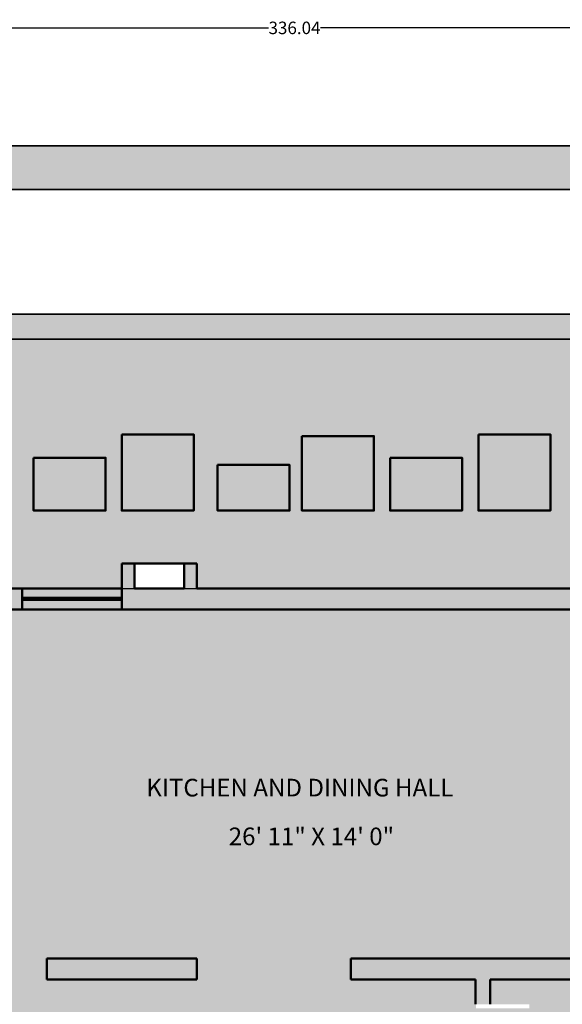
# Model space of a CAD drawing. Units: inches. Extents: x 925 to 2834, y 111 to 1355.
# Tile 17 of 25: x 1293 to 1553, y 882 to 1355. Entities that reach past the tile are written whole.
import ezdxf

# ---------------------------------------------------------------- set-up
doc = ezdxf.new("R2010")
doc.units = ezdxf.units.IN
doc.header["$MEASUREMENT"] = 0
for name, color, linetype, lineweight in [('A-ANNO-DIMS', 2, 'Continuous', 18), ('A-ANNO-TTLB', 7, 'Continuous', 35), ('A-AREA-IDEN', 7, 'Continuous', 18), ('A-FLOR-PATT', 252, 'Continuous', 13), ('A-GLAZ', 3, 'Continuous', 25), ('A-WALL', 7, 'Continuous', 50), ('A-WALL-PATT', 8, 'Continuous', 13)]:
    doc.layers.add(name, color=color, linetype=linetype, lineweight=lineweight)
doc.styles.get("Standard").update_dxf_attribs({"font": 'arial.ttf'})
doc.dimstyles.get("Standard").update_dxf_attribs({"dimtxt": 6, "dimasz": 3, "dimexe": 0.18, "dimexo": 0.0625, "dimgap": 0.09, "dimtad": 0, "dimtih": 1, "dimtoh": 1, "dimdec": 1, "dimzin": 0, "dimdsep": 46, "dimlunit": 3, "dimtxsty": 'Standard', "dimblk": 'ARCHTICK', "dimcen": 0.09, "dimadec": 0, "dimazin": 0, "dimtfac": 1, "dimtdec": 1, "dimtofl": 0, "dimtmove": 0, "dimatfit": 3, "dimfxl": 1, "dimtolj": 1, "dimtzin": 0, "dimarcsym": 0})

# ---------------------------------------------------------------- blocks, each defined once
blk = doc.blocks.new('_ArchTick')
at = {"color": 0, "linetype": 'ByBlock', "const_width": 0.15}
blk.add_lwpolyline([(-0.5, -0.5), (0.5, 0.5)], dxfattribs=at)
blk = doc.blocks.new('*D16')
at = {"layer": 'A-ANNO-DIMS', "color": 0, "lineweight": -2, "transparency": 16777216}
for p, q in [((1256.67, 1081.65), (1256.67, 1351.49)), ((1256.67, 1351.31), (1412.16, 1351.31)), ((1592.71, 1351.31), (1437.22, 1351.31)), ((1592.71, 1071.65), (1592.71, 1351.49))]:
    blk.add_line(p, q, dxfattribs=at)
at = {"layer": 'Defpoints', "color": 0, "transparency": 16777216}
for p in [(1592.71, 1351.31), (1256.67, 1081.59), (1592.71, 1071.59)]:
    blk.add_point(p, dxfattribs=at)
at = {"layer": 'A-ANNO-DIMS', "color": 0, "lineweight": -2, "transparency": 16777216, "xscale": 3, "yscale": 3, "zscale": 3, "rotation": 180}
blk.add_blockref('_ArchTick', (1256.67, 1351.31), dxfattribs=at)
at = {"layer": 'A-ANNO-DIMS', "color": 0, "lineweight": -2, "transparency": 16777216, "xscale": 3, "yscale": 3, "zscale": 3}
blk.add_blockref('_ArchTick', (1592.71, 1351.31), dxfattribs=at)
at = {"layer": 'A-ANNO-DIMS', "color": 0, "transparency": 16777216, "insert": (1424.69, 1351.31), "char_height": 6, "attachment_point": 5}
blk.add_mtext('\\A1;336.04', dxfattribs=at)

msp = doc.modelspace()

# ---------------------------------------------------------------- hatches: boundary and pattern name
at = {"layer": 'A-FLOR-PATT', "transparency": 33554605}
h = msp.add_hatch(color=256, dxfattribs=at)
h.dxf.hatch_style = 1
h.paths.add_polyline_path([(1931.688, 1294.5638), (991.7375, 1294.5638), (991.7375, 172.1134), (1931.688, 172.1134)])
h.paths.add_polyline_path([(1910.7128, 1273.5886), (1910.7128, 193.0886), (1012.7128, 193.0886), (1012.7128, 1273.5886)], flags=16)
h.paths.add_polyline_path([(1850.7128, 1213.5886), (1850.7128, 253.0886), (1072.7128, 253.0886), (1072.7128, 1213.5886)], flags=0)
h.paths.add_polyline_path([(1838.7128, 1201.5886), (1838.7128, 265.0886), (1084.7128, 265.0886), (1084.7128, 530.5886), (1084.7128, 1201.5886)], flags=0)
h.paths.add_polyline_path([(1547.6758, 1155.7396), (1547.6758, 1119.115), (1513.0687, 1119.115), (1513.0687, 1155.7396)], flags=0)
h.paths.add_polyline_path([(1600.1067, 1154.9439), (1634.7139, 1154.9439), (1634.7139, 1119.115), (1600.1067, 1119.115)], flags=0)
h.paths.add_polyline_path([(1505.2502, 1144.5358), (1505.2502, 1119.115), (1470.643, 1119.115), (1470.643, 1144.5358)], flags=0)
h.paths.add_polyline_path([(1559.1357, 1141.0962), (1593.7428, 1141.0962), (1593.7428, 1119.115), (1559.1357, 1119.115)], flags=0)
h.paths.add_polyline_path([(1462.8966, 1154.9439), (1462.8966, 1119.115), (1428.2895, 1119.115), (1428.2895, 1154.9439)], flags=0)
h.paths.add_polyline_path([(1642.4603, 1144.5358), (1677.0675, 1144.5358), (1677.0675, 1119.115), (1642.4603, 1119.115)], flags=0)
h.paths.add_polyline_path([(1422.3508, 1141.0962), (1422.3508, 1119.115), (1387.7436, 1119.115), (1387.7436, 1141.0962)], flags=0)
h.paths.add_polyline_path([(1684.8859, 1155.7396), (1719.4931, 1155.7396), (1719.4931, 1119.115), (1684.8859, 1119.115)], flags=0)
h.paths.add_polyline_path([(1718.7128, 1081.5886), (1718.7128, 1050.1249), (1715.7128, 1050.1249), (1715.7128, 1026.1249), (1715.7128, 1002.1249), (1718.7128, 1002.1249), (1730.7128, 1002.1249), (1730.7128, 998.1249), (1730.7128, 990.1249), (1730.7128, 986.1249), (1718.7128, 986.1249), (1718.7128, 893.5886), (1715.3735, 893.5886), (1715.3735, 891.5886), (1713.3735, 891.5886, 0.41421356), (1677.3735, 855.5886), (1713.3735, 855.5886), (1713.3735, 853.5886), (1715.3735, 853.5886), (1715.3735, 851.5886), (1718.7128, 851.5886), (1718.7128, 821.5865), (1734.4655, 821.5865), (1734.3735, 819.5886, -0.41421356), (1712.4415, 793.5886), (1712.4415, 791.5886), (1718.7128, 791.5886), (1718.7128, 717.5886), (1718.7128, 669.5886), (1732.7128, 669.5886), (1732.7128, 665.5886), (1732.7128, 641.5886), (1732.7128, 634.5886), (1732.7128, 610.5886), (1732.7128, 603.5886), (1718.7128, 603.5886), (1718.7128, 385.0886), (1434.2128, 385.0886), (1434.2128, 530.5886), (1410.2128, 530.5886), (1408.2128, 530.5886), (1408.2128, 532.5886, 0.41421356), (1372.2128, 568.5886), (1372.2128, 532.5886), (1370.2128, 532.5886), (1370.2128, 530.5886), (1368.2128, 530.5886), (1282.2128, 530.5886), (1210.2128, 530.5886), (1200.2128, 530.5886), (1200.2128, 542.1915), (1183.2307, 542.1915), (1183.2307, 546.1915), (1200.2128, 546.1915), (1200.2128, 572.1915), (1183.2307, 572.1915), (1183.2307, 576.1915), (1200.2128, 576.1915), (1200.2128, 727.5886), (1210.2128, 727.5886), (1234.2128, 727.5886), (1259.7128, 727.5886), (1259.7128, 775.5886), (1259.7128, 799.5886), (1259.7128, 847.5886), (1259.7128, 993.5872), (1259.7128, 1065.5872), (1259.7128, 1071.5886), (1219.6318, 1071.5886), (1219.6318, 1081.5886), (1084.7128, 1081.5886), (1084.7128, 1119.115), (1256.8974, 1119.115), (1256.8974, 1154.9439), (1291.5046, 1154.9439), (1291.5046, 1119.115), (1256.8974, 1119.115), (1256.6723, 1081.5886), (1293.7128, 1081.5886), (1341.7128, 1081.5886), (1341.7128, 1093.5886), (1347.7128, 1093.5886), (1371.7128, 1093.5886), (1377.7128, 1093.5886), (1377.7128, 1081.5886), (1668.7128, 1081.5886), (1668.7128, 1117.5886), (1675.7128, 1117.5886), (1711.7128, 1117.5886), (1718.7128, 1117.5886)], flags=0)
h.paths.add_polyline_path([(1376.2838, 1155.7396), (1376.2838, 1119.115), (1341.6766, 1119.115), (1341.6766, 1155.7396)], flags=0)
h.paths.add_polyline_path([(1341.7128, 1076.0886), (1293.7128, 1076.0886), (1293.7128, 1071.5886), (1269.7128, 1071.5886), (1269.7128, 1065.5872), (1266.7128, 1065.5872), (1266.7128, 1029.5872), (1265.7128, 1029.5872), (1265.7128, 993.5872), (1269.7128, 993.5872), (1269.7128, 903.5886), (1269.7128, 893.5886), (1269.7128, 847.5886), (1265.2128, 847.5886), (1265.2128, 799.5886), (1269.7128, 799.5886), (1269.7128, 775.5886), (1265.2128, 775.5886), (1265.2128, 727.5886), (1269.7128, 727.5886), (1444.2128, 727.5886), (1444.2128, 717.5886), (1234.2128, 717.5886), (1234.2128, 722.0886), (1210.2128, 722.0886), (1210.2128, 717.5886), (1210.2128, 540.5886), (1210.2128, 536.0886), (1282.2128, 536.0886), (1282.2128, 535.0886), (1210.2128, 535.0886), (1210.2128, 540.5886), (1210.2128, 717.5886), (1210.2128, 723.0886), (1234.2128, 723.0886), (1234.2128, 717.5886), (1444.2128, 717.5886), (1444.2128, 727.5886), (1269.7128, 727.5886), (1264.2128, 727.5886), (1264.2128, 775.5886), (1269.7128, 775.5886), (1269.7128, 799.5886), (1264.2128, 799.5886), (1264.2128, 847.5886), (1269.7128, 847.5886), (1269.7128, 893.5886), (1269.7128, 903.5886), (1269.7128, 993.5872), (1264.7128, 993.5872), (1264.7128, 1029.5872), (1265.7128, 1029.5872), (1265.7128, 1065.5872), (1269.7128, 1065.5872), (1269.7128, 1071.5886), (1293.7128, 1071.5886), (1293.7128, 1077.0886), (1341.7128, 1077.0886)], flags=0)
h.paths.add_polyline_path([(1730.9529, 1141.0962), (1765.5601, 1141.0962), (1765.5601, 1119.115), (1730.9529, 1119.115)], flags=0)
h.paths.add_polyline_path([(1333.8582, 1144.5358), (1333.8582, 1119.115), (1299.251, 1119.115), (1299.251, 1144.5358)], flags=0)
h.paths.add_polyline_path([(1592.7128, 968.5886), (1596.0342, 968.5886), (1602.7128, 968.5886), (1708.7128, 968.5886), (1708.7128, 903.5886), (1602.7128, 903.5886), (1602.7128, 938.5886), (1592.7128, 938.5886), (1592.7128, 903.5886), (1451.7128, 903.5886), (1451.7128, 893.5886), (1511.7128, 893.5886), (1511.7128, 881.5886), (1515.2128, 881.5886), (1518.7128, 881.5886), (1518.7128, 893.5886), (1592.7128, 893.5886), (1592.7128, 799.5886), (1518.7128, 799.5886), (1518.7128, 857.5886), (1511.7128, 857.5886), (1511.7128, 799.5886), (1511.7128, 772.0886), (1521.7128, 772.0886), (1521.7128, 792.5886), (1592.7128, 792.5886), (1592.7128, 727.5886), (1521.7128, 727.5886), (1521.7128, 748.0886), (1511.7128, 748.0886), (1511.7128, 717.5886), (1708.7128, 717.5886), (1714.2128, 717.5886), (1714.2128, 669.5886), (1708.7128, 669.5886), (1708.7128, 641.5886), (1492.2128, 641.5886), (1492.2128, 631.5886), (1621.2128, 631.5886), (1621.2128, 443.0886), (1625.7128, 443.0886), (1625.7128, 503.0886), (1625.7128, 507.5886), (1625.7128, 631.5886), (1708.7128, 631.5886), (1708.7128, 507.5886), (1655.7128, 507.5886), (1655.7128, 503.0886), (1708.7128, 503.0886), (1708.7128, 395.0886), (1625.7128, 395.0886), (1625.7128, 419.0886), (1621.2128, 419.0886), (1621.2128, 395.0886), (1482.2128, 395.0886), (1482.2128, 385.0886), (1434.2128, 385.0886), (1434.2128, 433.0886), (1444.2128, 433.0886), (1444.2128, 631.5886), (1450.2128, 631.5886), (1450.2128, 634.91), (1452.2128, 634.91), (1452.2128, 669.5886), (1454.2128, 669.5886, -0.40021217), (1490.1712, 635.3173), (1492.2128, 635.3173), (1492.2128, 641.5886), (1564.7128, 641.5886), (1564.7128, 677.5886), (1672.7128, 677.5886), (1672.7128, 681.5886), (1564.7128, 681.5886), (1564.7128, 717.5886), (1511.7128, 717.5886), (1511.7128, 748.0886), (1511.7128, 772.0886), (1511.7128, 799.5886), (1511.7128, 857.5886), (1511.8913, 857.5886), (1511.8913, 859.5886), (1515.6201, 859.5886, 0.41421356), (1537.552, 879.5886), (1513.552, 879.5886), (1511.8913, 879.5886), (1511.8913, 881.5886), (1511.7128, 881.5886), (1511.7128, 893.5886), (1451.7128, 893.5886), (1451.7128, 903.5886), (1592.7128, 903.5886), (1592.7128, 938.5886), (1592.7128, 940.5886), (1596.4415, 940.5886, 0.41421356), (1618.3735, 966.5886), (1594.3735, 966.5886), (1592.7128, 966.5886)], flags=0)
h.paths.add_polyline_path([(1377.7128, 903.5886), (1377.7128, 893.5886), (1305.7128, 893.5886), (1305.7128, 903.5886)], flags=0)
h.paths.add_polyline_path([(1708.7128, 821.5886), (1712.0342, 821.5886), (1712.0342, 819.5886), (1710.3735, 819.5886), (1708.7128, 819.5886)], flags=0)
h.paths.add_polyline_path([(1576.7128, 695.1992), (1575.5896, 693.6649), (1575.9687, 694.6994), (1575.4438, 695.1992), (1575.9687, 695.699), (1575.5896, 696.7335)], flags=0)
h.paths.add_polyline_path([(1565.9817, 662.3134), (1565.4568, 661.8136), (1565.8359, 660.7791), (1564.7128, 662.3134), (1565.8359, 663.8477), (1565.4568, 662.8132)], flags=0)
h.paths.add_polyline_path([(1444.2128, 433.0886), (1444.2128, 395.0886), (1482.2128, 395.0886), (1482.2128, 389.0886), (1438.2128, 389.0886), (1438.2128, 391.8608), (1438.2128, 433.0886)], flags=0)
h.paths.add_polyline_path([(1410.2128, 506.5886), (1410.2128, 289.0886), (1108.7128, 289.0886), (1108.7128, 506.5886)], flags=0)
h.paths.add_polyline_path([(1612.3153, 838.3016), (1680.4151, 838.3016), (1680.4151, 851.3131), (1612.3153, 851.3131)], flags=8)
h.paths.add_polyline_path([(1208.3174, 395.0436), (1282.1017, 395.0436), (1282.1017, 408.0552), (1208.3174, 408.0552)], flags=8)
h.paths.add_polyline_path([(1291.8049, 598.7427), (1369.8017, 598.7427), (1369.8017, 611.7542), (1291.8049, 611.7542)], flags=8)
h.paths.add_polyline_path([(1119.679, 917.3022), (1191.0817, 917.3022), (1191.0817, 930.3137), (1119.679, 930.3137)], flags=8)
h.paths.add_polyline_path([(1332.2261, 815.9808), (1410.2258, 815.9808), (1410.2258, 829.001), (1332.2261, 829.001)], flags=8)
h.paths.add_polyline_path([(1390.9013, 955.8158), (1475.4981, 955.8158), (1475.4981, 968.8273), (1390.9013, 968.8273)], flags=8)
h.paths.add_polyline_path([(1620.3436, 998.9325), (1688.4434, 998.9325), (1688.4434, 1011.944), (1620.3436, 1011.944)], flags=8)
h.paths.add_polyline_path([(1620.3436, 914.1039), (1691.7405, 914.1039), (1691.7405, 927.1155), (1620.3436, 927.1155)], flags=8)
h.paths.add_polyline_path([(1521.4542, 816.005), (1589.5569, 816.005), (1589.5569, 829.0253), (1521.4542, 829.0253)], flags=8)
h.paths.add_polyline_path([(1528.524, 740.3497), (1602.3082, 740.3497), (1602.3082, 753.3613), (1528.524, 753.3613)], flags=8)
h.paths.add_polyline_path([(1627.6094, 762.6128), (1702.3091, 762.6128), (1702.3091, 775.6244), (1627.6094, 775.6244)], flags=8)
h.paths.add_polyline_path([(1610.5442, 657.2751), (1684.3284, 657.2751), (1684.3284, 670.2867), (1610.5442, 670.2867)], flags=8)
h.paths.add_polyline_path([(1636.6983, 519.472), (1711.3981, 519.472), (1711.3981, 532.4835), (1636.6983, 532.4835)], flags=8)
h.paths.add_polyline_path([(1616.8577, 424.8539), (1694.8545, 424.8539), (1694.8545, 437.8654), (1616.8577, 437.8654)], flags=8)
h.paths.add_polyline_path([(1506.1456, 460.8838), (1579.9299, 460.8838), (1579.9299, 473.8953), (1506.1456, 473.8953)], flags=8)
h.paths.add_polyline_path([(1624.6119, 784.6011), (1696.9185, 784.6011), (1696.9185, 797.7864), (1624.6119, 797.7864)], flags=8)
h.paths.add_polyline_path([(1606.3732, 854.2194), (1683.3039, 854.2194), (1683.3039, 867.4048), (1606.3732, 867.4048)], flags=8)
h.paths.add_polyline_path([(1127.8008, 940.3581), (1165.1637, 940.3581), (1165.1637, 953.5348), (1127.8008, 953.5348)], flags=8)
h.paths.add_polyline_path([(1620.8657, 1019.4968), (1677.3447, 1019.4968), (1677.3447, 1032.6735), (1620.8657, 1032.6735)], flags=8)
h.paths.add_polyline_path([(1620.8643, 930.1821), (1703.0564, 930.1821), (1703.0564, 943.3675), (1620.8643, 943.3675)], flags=8)
h.paths.add_polyline_path([(1324.5702, 836.8338), (1408.0892, 836.8338), (1408.0892, 850.0191), (1324.5702, 850.0191)], flags=8)
h.paths.add_polyline_path([(1281.6584, 622.8885), (1383.6213, 622.8885), (1383.6213, 636.0739), (1281.6584, 636.0739)], flags=8)
h.paths.add_polyline_path([(1210.6721, 416.7893), (1269.1299, 416.7893), (1269.1299, 429.9747), (1210.6721, 429.9747)], flags=8)
h.paths.add_polyline_path([(1507.8264, 477.4836), (1586.7329, 477.4836), (1586.7329, 490.669), (1507.8264, 490.669)], flags=8)
h.paths.add_polyline_path([(1643.6238, 443.8135), (1696.6696, 443.8135), (1696.6696, 456.5643), (1643.6238, 456.5643)], flags=8)
h.paths.add_polyline_path([(1647.2466, 540.5638), (1693.1825, 540.5638), (1693.1825, 553.7491), (1647.2466, 553.7491)], flags=8)
h.paths.add_polyline_path([(1626.0633, 668.5064), (1673.3174, 668.5064), (1673.3174, 681.6831), (1626.0633, 681.6831)], flags=8)
h.paths.add_polyline_path([(1538.2915, 830.7872), (1567.5942, 830.7872), (1567.5942, 843.5293), (1538.2915, 843.5293)], flags=8)
h.paths.add_polyline_path([(1530.9338, 754.0477), (1559.576, 754.0477), (1559.576, 766.7898), (1530.9338, 766.7898)], flags=8)
h.paths.add_polyline_path([(1351.2461, 979.2309), (1513.8919, 979.2309), (1513.8919, 992.4076), (1351.2461, 992.4076)], flags=8)
at = {"layer": 'A-FLOR-PATT'}
h = msp.add_hatch(color=256, dxfattribs=at)
h.dxf.hatch_style = 1
h.paths.add_polyline_path([(1850.7128, 1213.5886), (1072.7128, 1213.5886), (1072.7128, 253.0886), (1850.7128, 253.0886)])
h.paths.add_polyline_path([(1084.7128, 1201.5886), (1838.7128, 1201.5886), (1838.7128, 265.0886), (1084.7128, 265.0886)], flags=16)
h.paths.add_polyline_path([(1183.2307, 576.1915), (1200.2128, 576.1915), (1200.2128, 727.5886), (1210.2128, 727.5886), (1234.2128, 727.5886), (1259.7128, 727.5886), (1259.7128, 775.5886), (1259.7128, 799.5886), (1259.7128, 847.5886), (1259.7128, 993.5872), (1259.7128, 1065.5872), (1259.7128, 1071.5886), (1219.6318, 1071.5886), (1219.6318, 1081.5886), (1293.7128, 1081.5886), (1341.7128, 1081.5886), (1341.7128, 1093.5886), (1347.7128, 1093.5886), (1347.7128, 1081.5886), (1371.7128, 1081.5886), (1371.7128, 1093.5886), (1377.7128, 1093.5886), (1377.7128, 1081.5886), (1668.7128, 1081.5886), (1668.7128, 1117.5886), (1675.7128, 1117.5886), (1675.7128, 1081.5886), (1711.7128, 1081.5886), (1711.7128, 1117.5886), (1718.7128, 1117.5886), (1718.7128, 1081.5886), (1718.7128, 1050.1249), (1715.7128, 1050.1249), (1715.7128, 1026.1249), (1715.7128, 1002.1249), (1718.7128, 1002.1249), (1730.7128, 1002.1249), (1730.7128, 998.1249), (1730.7128, 990.1249), (1730.7128, 986.1249), (1718.7128, 986.1249), (1718.7128, 893.5886), (1715.3735, 893.5886), (1715.3735, 891.5886), (1713.3735, 891.5886, 0.41421356), (1677.3735, 855.5886), (1713.3735, 855.5886), (1713.3735, 853.5886), (1715.3735, 853.5886), (1715.3735, 851.5886), (1718.7128, 851.5886), (1718.7128, 821.5865), (1734.4655, 821.5865), (1734.3735, 819.5886, -0.41421356), (1712.4415, 793.5886), (1712.4415, 791.5886), (1718.7128, 791.5886), (1718.7128, 717.5886), (1718.7128, 669.5886), (1732.7128, 669.5886), (1732.7128, 665.5886), (1732.7128, 641.5886), (1732.7128, 634.5886), (1732.7128, 610.5886), (1732.7128, 603.5886), (1718.7128, 603.5886), (1718.7128, 385.0886), (1434.2128, 385.0886), (1434.2128, 433.0886), (1434.2128, 530.5886), (1410.2128, 530.5886), (1408.2128, 530.5886), (1408.2128, 532.5886, 0.41421356), (1372.2128, 568.5886), (1372.2128, 532.5886), (1370.2128, 532.5886), (1370.2128, 530.5886), (1368.2128, 530.5886), (1282.2128, 530.5886), (1210.2128, 530.5886), (1200.2128, 530.5886), (1200.2128, 542.1915), (1183.2307, 542.1915), (1183.2307, 546.1915), (1200.2128, 546.1915), (1200.2128, 572.1915), (1183.2307, 572.1915)], flags=0)
h.paths.add_polyline_path([(1210.2128, 717.5886), (1210.2128, 723.0886), (1234.2128, 723.0886), (1234.2128, 717.5886), (1444.2128, 717.5886), (1444.2128, 727.5886), (1269.7128, 727.5886), (1264.2128, 727.5886), (1264.2128, 775.5886), (1269.7128, 775.5886), (1269.7128, 799.5886), (1264.2128, 799.5886), (1264.2128, 847.5886), (1269.7128, 847.5886), (1269.7128, 893.5886), (1269.7128, 903.5886), (1269.7128, 993.5872), (1264.7128, 993.5872), (1264.7128, 1029.5872), (1265.7128, 1029.5872), (1265.7128, 1065.5872), (1269.7128, 1065.5872), (1269.7128, 1071.5886), (1293.7128, 1071.5886), (1293.7128, 1077.0886), (1341.7128, 1077.0886), (1341.7128, 1076.0886), (1293.7128, 1076.0886), (1293.7128, 1071.5886), (1269.7128, 1071.5886), (1269.7128, 1065.5872), (1266.7128, 1065.5872), (1266.7128, 1029.5872), (1265.7128, 1029.5872), (1265.7128, 993.5872), (1269.7128, 993.5872), (1269.7128, 903.5886), (1269.7128, 893.5886), (1269.7128, 847.5886), (1265.2128, 847.5886), (1265.2128, 799.5886), (1269.7128, 799.5886), (1269.7128, 775.5886), (1265.2128, 775.5886), (1265.2128, 727.5886), (1269.7128, 727.5886), (1444.2128, 727.5886), (1444.2128, 717.5886), (1234.2128, 717.5886), (1234.2128, 722.0886), (1210.2128, 722.0886), (1210.2128, 717.5886), (1210.2128, 540.5886), (1210.2128, 536.0886), (1282.2128, 536.0886), (1282.2128, 535.0886), (1210.2128, 535.0886), (1210.2128, 540.5886)], flags=0)
h.paths.add_polyline_path([(1450.2128, 634.91), (1452.2128, 634.91), (1452.2128, 669.5886), (1454.2128, 669.5886, -0.40021217), (1490.1712, 635.3173), (1492.2128, 635.3173), (1492.2128, 641.5886), (1564.7128, 641.5886), (1564.7128, 677.5886), (1672.7128, 677.5886), (1672.7128, 681.5886), (1564.7128, 681.5886), (1564.7128, 717.5886), (1511.7128, 717.5886), (1511.7128, 748.0886), (1511.7128, 772.0886), (1511.7128, 799.5886), (1511.7128, 857.5886), (1511.8913, 857.5886), (1511.8913, 859.5886), (1515.6201, 859.5886, 0.41421356), (1537.552, 879.5886), (1513.552, 879.5886), (1511.8913, 879.5886), (1511.8913, 881.5886), (1511.7128, 881.5886), (1511.7128, 893.5886), (1451.7128, 893.5886), (1451.7128, 903.5886), (1592.7128, 903.5886), (1592.7128, 938.5886), (1592.7128, 940.5886), (1596.4415, 940.5886, 0.41421356), (1618.3735, 966.5886), (1594.3735, 966.5886), (1592.7128, 966.5886), (1592.7128, 968.5886), (1596.0342, 968.5886), (1602.7128, 968.5886), (1708.7128, 968.5886), (1708.7128, 903.5886), (1602.7128, 903.5886), (1602.7128, 938.5886), (1592.7128, 938.5886), (1592.7128, 903.5886), (1451.7128, 903.5886), (1451.7128, 893.5886), (1511.7128, 893.5886), (1511.7128, 881.5886), (1518.7128, 881.5886), (1518.7128, 893.5886), (1592.7128, 893.5886), (1592.7128, 799.5886), (1518.7128, 799.5886), (1518.7128, 857.5886), (1511.7128, 857.5886), (1511.7128, 799.5886), (1511.7128, 772.0886), (1521.7128, 772.0886), (1521.7128, 792.5886), (1592.7128, 792.5886), (1592.7128, 727.5886), (1521.7128, 727.5886), (1521.7128, 748.0886), (1511.7128, 748.0886), (1511.7128, 717.5886), (1708.7128, 717.5886), (1714.2128, 717.5886), (1714.2128, 669.5886), (1708.7128, 669.5886), (1708.7128, 641.5886), (1492.2128, 641.5886), (1492.2128, 631.5886), (1621.2128, 631.5886), (1621.2128, 443.0886), (1625.7128, 443.0886), (1625.7128, 503.0886), (1625.7128, 507.5886), (1625.7128, 631.5886), (1708.7128, 631.5886), (1708.7128, 507.5886), (1655.7128, 507.5886), (1655.7128, 503.0886), (1708.7128, 503.0886), (1708.7128, 395.0886), (1625.7128, 395.0886), (1625.7128, 419.0886), (1621.2128, 419.0886), (1621.2128, 395.0886), (1482.2128, 395.0886), (1482.2128, 389.0886), (1438.2128, 389.0886), (1438.2128, 391.8608), (1438.2128, 433.0886), (1444.2128, 433.0886), (1444.2128, 631.5886), (1450.2128, 631.5886)], flags=0)
h.paths.add_polyline_path([(1444.2128, 433.0886), (1444.2128, 395.0886), (1482.2128, 395.0886), (1482.2128, 391.0886), (1440.2128, 391.0886), (1440.2128, 391.8608), (1440.2128, 433.0886)], flags=0)
h.paths.add_polyline_path([(1305.7128, 893.5886), (1305.7128, 903.5886), (1377.7128, 903.5886), (1377.7128, 893.5886)], flags=0)
h.paths.add_polyline_path([(1564.7128, 662.3134), (1565.8359, 663.8477), (1565.4568, 662.8132), (1565.9817, 662.3134), (1565.4568, 661.8136), (1565.8359, 660.7791)], flags=0)
h.paths.add_polyline_path([(1575.4438, 695.1992), (1575.9687, 695.699), (1575.5896, 696.7335), (1576.7128, 695.1992), (1575.5896, 693.6649), (1575.9687, 694.6994)], flags=0)
h.paths.add_polyline_path([(1708.7128, 821.5886), (1712.0342, 821.5886), (1712.0342, 819.5886), (1710.3735, 819.5886), (1708.7128, 819.5886)], flags=0)
at = {"layer": 'A-FLOR-PATT', "transparency": 33554554}
h = msp.add_hatch(color=256, dxfattribs=at)
h.dxf.hatch_style = 1
h.paths.add_polyline_path([(1838.7128, 1201.5886), (1084.7128, 1201.5886), (1084.7128, 1119.115), (1256.8974, 1119.115), (1256.8974, 1154.9439), (1291.5046, 1154.9439), (1291.5046, 1119.115), (1256.8974, 1119.115), (1256.6723, 1081.5886), (1293.7128, 1081.5886), (1341.7128, 1081.5886), (1341.7128, 1093.5886), (1347.7128, 1093.5886), (1371.7128, 1093.5886), (1377.7128, 1093.5886), (1377.7128, 1081.5886), (1668.7128, 1081.5886), (1668.7128, 1117.5886), (1675.7128, 1117.5886), (1711.7128, 1117.5886), (1718.7128, 1117.5886), (1718.7128, 1081.5886), (1838.7128, 1081.5886)])
h.paths.add_polyline_path([(1299.251, 1144.5358), (1333.8582, 1144.5358), (1333.8582, 1119.115), (1299.251, 1119.115)], flags=16)
h.paths.add_polyline_path([(1341.6766, 1155.7396), (1376.2838, 1155.7396), (1376.2838, 1119.115), (1341.6766, 1119.115)], flags=16)
h.paths.add_polyline_path([(1387.7436, 1141.0962), (1422.3508, 1141.0962), (1422.3508, 1119.115), (1387.7436, 1119.115)], flags=16)
h.paths.add_polyline_path([(1428.2895, 1154.9439), (1462.8966, 1154.9439), (1462.8966, 1119.115), (1428.2895, 1119.115)], flags=16)
h.paths.add_polyline_path([(1470.643, 1144.5358), (1505.2502, 1144.5358), (1505.2502, 1119.115), (1470.643, 1119.115)], flags=16)
h.paths.add_polyline_path([(1513.0687, 1155.7396), (1547.6758, 1155.7396), (1547.6758, 1119.115), (1513.0687, 1119.115)], flags=16)
h.paths.add_polyline_path([(1559.1357, 1141.0962), (1593.7428, 1141.0962), (1593.7428, 1119.115), (1559.1357, 1119.115)], flags=16)
h.paths.add_polyline_path([(1600.1067, 1154.9439), (1634.7139, 1154.9439), (1634.7139, 1119.115), (1600.1067, 1119.115)], flags=16)
h.paths.add_polyline_path([(1642.4603, 1144.5358), (1677.0675, 1144.5358), (1677.0675, 1119.115), (1642.4603, 1119.115)], flags=16)
h.paths.add_polyline_path([(1684.8859, 1155.7396), (1719.4931, 1155.7396), (1719.4931, 1119.115), (1684.8859, 1119.115)], flags=16)
h.paths.add_polyline_path([(1730.9529, 1141.0962), (1765.5601, 1141.0962), (1765.5601, 1119.115), (1730.9529, 1119.115)], flags=16)
at = {"layer": 'A-FLOR-PATT', "transparency": 33554661}
h = msp.add_hatch(color=256, dxfattribs=at)
h.dxf.hatch_style = 1
h.paths.add_polyline_path([(1291.5046, 1154.9439), (1256.8974, 1154.9439), (1256.8974, 1119.115), (1291.5046, 1119.115)])
h.paths.add_polyline_path([(1333.8582, 1144.5358), (1299.251, 1144.5358), (1299.251, 1119.115), (1333.8582, 1119.115)])
h.paths.add_polyline_path([(1376.2838, 1155.7396), (1341.6766, 1155.7396), (1341.6766, 1119.115), (1376.2838, 1119.115)])
h.paths.add_polyline_path([(1422.3508, 1141.0962), (1387.7436, 1141.0962), (1387.7436, 1119.115), (1422.3508, 1119.115)])
h.paths.add_polyline_path([(1462.8966, 1154.9439), (1428.2895, 1154.9439), (1428.2895, 1119.115), (1462.8966, 1119.115)])
h.paths.add_polyline_path([(1505.2502, 1144.5358), (1470.643, 1144.5358), (1470.643, 1119.115), (1505.2502, 1119.115)])
h.paths.add_polyline_path([(1547.6758, 1155.7396), (1513.0687, 1155.7396), (1513.0687, 1119.115), (1547.6758, 1119.115)])
h.paths.add_polyline_path([(1593.7428, 1141.0962), (1559.1357, 1141.0962), (1559.1357, 1119.115), (1593.7428, 1119.115)])
h.paths.add_polyline_path([(1634.7139, 1154.9439), (1600.1067, 1154.9439), (1600.1067, 1119.115), (1634.7139, 1119.115)])
h.paths.add_polyline_path([(1677.0675, 1144.5358), (1642.4603, 1144.5358), (1642.4603, 1119.115), (1677.0675, 1119.115)])
h.paths.add_polyline_path([(1719.4931, 1155.7396), (1684.8859, 1155.7396), (1684.8859, 1119.115), (1719.4931, 1119.115)])
h.paths.add_polyline_path([(1765.5601, 1141.0962), (1730.9529, 1141.0962), (1730.9529, 1119.115), (1765.5601, 1119.115)])
at = {"layer": 'A-FLOR-PATT'}
h = msp.add_hatch(color=256, dxfattribs=at)
h.dxf.hatch_style = 1
h.paths.add_polyline_path([(1718.7128, 603.5886), (1708.7128, 603.5886), (1708.7128, 507.5886), (1655.7128, 507.5886), (1655.7128, 503.0886), (1708.7128, 503.0886), (1708.7128, 395.0886), (1625.7128, 395.0886), (1625.7128, 419.0886), (1621.2128, 419.0886), (1621.2128, 395.0886), (1482.2128, 395.0886), (1482.2128, 385.0886), (1718.7128, 385.0886)])
h.paths.add_polyline_path([(1625.7128, 631.5886), (1708.7128, 631.5886), (1708.7128, 603.5886), (1718.7128, 603.5886), (1732.7128, 603.5886), (1732.7128, 610.5886), (1715.7128, 610.5886), (1715.7128, 634.5886), (1732.7128, 634.5886), (1732.7128, 641.5886), (1715.7128, 641.5886), (1715.7128, 665.5886), (1732.7128, 665.5886), (1732.7128, 669.5886), (1708.7128, 669.5886), (1708.7128, 641.5886), (1492.2128, 641.5886), (1492.2128, 631.5886), (1621.2128, 631.5886), (1621.2128, 443.0886), (1625.7128, 443.0886), (1625.7128, 503.0886), (1625.7128, 507.5886)])
h.paths.add_polyline_path([(1718.7128, 851.5886), (1708.7128, 851.5886), (1708.7128, 828.5886), (1602.7128, 828.5886), (1602.7128, 893.5886), (1708.7128, 893.5886), (1718.7128, 893.5886), (1718.7128, 986.1249), (1730.7128, 986.1249), (1730.7128, 990.1249), (1718.7128, 990.1249), (1718.7128, 998.1249), (1730.7128, 998.1249), (1730.7128, 1002.1249), (1718.7128, 1002.1249), (1708.7128, 1002.1249), (1708.7128, 975.5886), (1602.7128, 975.5886), (1602.7128, 1011.5886), (1592.7128, 1011.5886), (1592.7128, 968.5886), (1596.0342, 968.5886), (1602.7128, 968.5886), (1708.7128, 968.5886), (1708.7128, 903.5886), (1602.7128, 903.5886), (1602.7128, 938.5886), (1592.7128, 938.5886), (1592.7128, 903.5886), (1451.7128, 903.5886), (1451.7128, 893.5886), (1511.7128, 893.5886), (1511.7128, 881.5886), (1515.2128, 881.5886), (1518.7128, 881.5886), (1518.7128, 893.5886), (1592.7128, 893.5886), (1592.7128, 799.5886), (1518.7128, 799.5886), (1518.7128, 857.5886), (1511.7128, 857.5886), (1511.7128, 799.5886), (1511.7128, 772.0886), (1521.7128, 772.0886), (1521.7128, 792.5886), (1592.7128, 792.5886), (1592.7128, 727.5886), (1521.7128, 727.5886), (1521.7128, 748.0886), (1511.7128, 748.0886), (1511.7128, 717.5886), (1708.7128, 717.5886), (1718.7128, 717.5886), (1718.7128, 727.5886), (1718.7128, 791.5886), (1708.7128, 791.5886), (1708.7128, 727.5886), (1602.7128, 727.5886), (1602.7128, 821.5886), (1708.7128, 821.5886), (1712.0342, 821.5886), (1718.7128, 821.5886)])
h.paths.add_polyline_path([(1718.7128, 1081.5886), (1718.7128, 1117.5886), (1711.7128, 1117.5886), (1711.7128, 1081.5886), (1675.7128, 1081.5886), (1675.7128, 1117.5886), (1668.7128, 1117.5886), (1668.7128, 1081.5886), (1377.7128, 1081.5886), (1377.7128, 1093.5886), (1371.7128, 1093.5886), (1371.7128, 1081.5886), (1347.7128, 1081.5886), (1347.7128, 1093.5886), (1341.7128, 1093.5886), (1341.7128, 1081.5886), (1341.7128, 1071.5886), (1592.7128, 1071.5886), (1592.7128, 1035.5886), (1602.7128, 1035.5886), (1602.7128, 1071.5886), (1708.7128, 1071.5886), (1708.7128, 1050.1249), (1718.7128, 1050.1249)])
h.paths.add_polyline_path([(1293.7128, 1081.5886), (1219.6318, 1081.5886), (1219.6318, 1071.5886), (1259.7128, 1071.5886), (1259.7128, 1065.5872), (1269.7128, 1065.5872), (1269.7128, 1071.5886), (1293.7128, 1071.5886)])
h.paths.add_polyline_path([(1269.7128, 903.5886), (1269.7128, 993.5872), (1259.7128, 993.5872), (1259.7128, 847.5886), (1269.7128, 847.5886), (1269.7128, 893.5886)])
h.paths.add_polyline_path([(1377.7128, 903.5886), (1305.7128, 903.5886), (1305.7128, 893.5886), (1377.7128, 893.5886)])
h.paths.add_polyline_path([(1444.2128, 727.5886), (1269.7128, 727.5886), (1259.7128, 727.5886), (1234.2128, 727.5886), (1234.2128, 717.5886), (1444.2128, 717.5886)])
h.paths.add_polyline_path([(1269.7128, 799.5886), (1259.7128, 799.5886), (1259.7128, 775.5886), (1269.7128, 775.5886)])
h.paths.add_polyline_path([(1444.2128, 631.5886), (1450.2128, 631.5886), (1450.2128, 634.91), (1450.2128, 641.5886), (1434.2128, 641.5886), (1434.2128, 540.5886), (1410.2128, 540.5886), (1410.2128, 530.5886), (1434.2128, 530.5886), (1434.2128, 433.0886), (1444.2128, 433.0886)])
h.paths.add_polyline_path([(1368.2128, 533.91), (1368.2128, 540.5886), (1282.2128, 540.5886), (1282.2128, 530.5886), (1368.2128, 530.5886)])
h.paths.add_polyline_path([(1210.2128, 717.5886), (1210.2128, 727.5886), (1200.2128, 727.5886), (1200.2128, 576.1915), (1183.2307, 576.1915), (1183.2307, 572.1915), (1200.2128, 572.1915), (1200.2128, 546.1915), (1183.2307, 546.1915), (1183.2307, 542.1915), (1200.2128, 542.1915), (1200.2128, 530.5886), (1210.2128, 530.5886), (1210.2128, 540.5886)])
at = {"layer": 'A-FLOR-PATT', "transparency": 33554605}
h = msp.add_hatch(color=256, dxfattribs=at)
h.dxf.hatch_style = 1
h.paths.add_polyline_path([(1592.7128, 938.5886), (1592.7128, 940.5886), (1596.4415, 940.5886, 0.41421356), (1618.3735, 966.5886), (1594.3735, 966.5886), (1592.7128, 966.5886), (1592.7128, 968.5886), (1592.7128, 1011.5886), (1602.7128, 1011.5886), (1602.7128, 975.5886), (1708.7128, 975.5886), (1708.7128, 1002.1249), (1711.7128, 1002.1249), (1711.7128, 1026.1249), (1711.7128, 1050.1249), (1708.7128, 1050.1249), (1708.7128, 1071.5886), (1602.7128, 1071.5886), (1602.7128, 1035.5886), (1592.7128, 1035.5886), (1592.7128, 1071.5886), (1341.7128, 1071.5886), (1293.7128, 1071.5886), (1269.7128, 1071.5886), (1269.7128, 1065.5872), (1269.7128, 993.5872), (1269.7128, 903.5886), (1269.7128, 893.5886), (1269.7128, 847.5886), (1269.7128, 799.5886), (1269.7128, 775.5886), (1269.7128, 727.5886), (1444.2128, 727.5886), (1444.2128, 717.5886), (1234.2128, 717.5886), (1210.2128, 717.5886), (1210.2128, 540.5886), (1282.2128, 540.5886), (1368.2128, 540.5886), (1368.2128, 533.91), (1370.2128, 533.91), (1370.2128, 568.5886), (1372.2128, 568.5886, -0.40021217), (1408.1712, 534.3173), (1410.2128, 534.3173), (1410.2128, 540.5886), (1434.2128, 540.5886), (1434.2128, 641.5886), (1450.2128, 641.5886), (1450.2128, 634.91), (1452.2128, 634.91), (1452.2128, 669.5886), (1454.2128, 669.5886, -0.40021217), (1490.1712, 635.3173), (1492.2128, 635.3173), (1492.2128, 641.5886), (1564.7128, 641.5886), (1564.7128, 677.5886), (1672.7128, 677.5886), (1672.7128, 681.5886), (1564.7128, 681.5886), (1564.7128, 717.5886), (1511.7128, 717.5886), (1511.7128, 748.0886), (1511.7128, 772.0886), (1511.7128, 799.5886), (1511.7128, 857.5886), (1511.8913, 857.5886), (1511.8913, 859.5886), (1515.6201, 859.5886, 0.41421356), (1537.552, 879.5886), (1513.552, 879.5886), (1511.8913, 879.5886), (1511.8913, 881.5886), (1511.7128, 881.5886), (1511.7128, 893.5886), (1451.7128, 893.5886), (1451.7128, 903.5886), (1592.7128, 903.5886)])
h.paths.add_polyline_path([(1377.7128, 903.5886), (1377.7128, 893.5886), (1305.7128, 893.5886), (1305.7128, 903.5886)], flags=16)
h.paths.add_polyline_path([(1592.7128, 893.5886), (1518.7128, 893.5886), (1518.7128, 881.5865), (1537.6441, 881.5865), (1537.552, 879.5886, -0.41421356), (1515.6201, 859.5886), (1515.6201, 857.5886), (1518.7128, 857.5886), (1518.7128, 799.5886), (1592.7128, 799.5886)], flags=17)
h.paths.add_polyline_path([(1291.8049, 598.7427), (1369.8017, 598.7427), (1369.8017, 611.7542), (1291.8049, 611.7542)], flags=24)
h.paths.add_polyline_path([(1332.2261, 815.9808), (1410.2258, 815.9808), (1410.2258, 829.001), (1332.2261, 829.001)], flags=24)
h.paths.add_polyline_path([(1390.9013, 955.8158), (1475.4981, 955.8158), (1475.4981, 968.8273), (1390.9013, 968.8273)], flags=24)
h.paths.add_polyline_path([(1620.3436, 998.9325), (1688.4434, 998.9325), (1688.4434, 1011.944), (1620.3436, 1011.944)], flags=24)
h.paths.add_polyline_path([(1620.8657, 1019.4968), (1677.3447, 1019.4968), (1677.3447, 1032.6735), (1620.8657, 1032.6735)], flags=24)
h.paths.add_polyline_path([(1324.5702, 836.8338), (1408.0892, 836.8338), (1408.0892, 850.0191), (1324.5702, 850.0191)], flags=24)
h.paths.add_polyline_path([(1281.6584, 622.8885), (1383.6213, 622.8885), (1383.6213, 636.0739), (1281.6584, 636.0739)], flags=24)
h.paths.add_polyline_path([(1626.0633, 668.5064), (1673.3174, 668.5064), (1673.3174, 681.6831), (1626.0633, 681.6831)], flags=25)
h.paths.add_polyline_path([(1351.2461, 979.2309), (1513.8919, 979.2309), (1513.8919, 992.4076), (1351.2461, 992.4076)], flags=24)
h.paths.add_polyline_path([(1521.4542, 816.005), (1589.5569, 816.005), (1589.5569, 829.0253), (1521.4542, 829.0253)], flags=24)
h.paths.add_polyline_path([(1538.2915, 830.7872), (1567.5942, 830.7872), (1567.5942, 843.5293), (1538.2915, 843.5293)], flags=24)
h.paths.add_polyline_path([(1636.6983, 519.472), (1711.3981, 519.472), (1711.3981, 532.4835), (1636.6983, 532.4835)], flags=9)
h.paths.add_polyline_path([(1616.8577, 424.8539), (1694.8545, 424.8539), (1694.8545, 437.8654), (1616.8577, 437.8654)], flags=9)
h.paths.add_polyline_path([(1506.1456, 460.8838), (1579.9299, 460.8838), (1579.9299, 473.8953), (1506.1456, 473.8953)], flags=9)
h.paths.add_polyline_path([(1606.3732, 854.2194), (1683.3039, 854.2194), (1683.3039, 867.4048), (1606.3732, 867.4048)], flags=25)
h.paths.add_polyline_path([(1507.8264, 477.4836), (1586.7329, 477.4836), (1586.7329, 490.669), (1507.8264, 490.669)], flags=9)
h.paths.add_polyline_path([(1643.6238, 443.8135), (1696.6696, 443.8135), (1696.6696, 456.5643), (1643.6238, 456.5643)], flags=9)
h.paths.add_polyline_path([(1647.2466, 540.5638), (1693.1825, 540.5638), (1693.1825, 553.7491), (1647.2466, 553.7491)], flags=25)
h = msp.add_hatch(color=256, dxfattribs=at)
h.dxf.hatch_style = 1
h.paths.add_polyline_path([(1200.2128, 727.5886), (1084.7128, 727.5886), (1084.7128, 530.5886), (1200.2128, 530.5886), (1200.2128, 542.1915), (1183.2307, 542.1915), (1183.2307, 546.1915), (1200.2128, 546.1915), (1200.2128, 572.1915), (1183.2307, 572.1915), (1183.2307, 576.1915), (1200.2128, 576.1915)])
h.paths.add_polyline_path([(1612.3153, 838.3016), (1680.4151, 838.3016), (1680.4151, 851.3131), (1612.3153, 851.3131)], flags=9)
h.paths.add_polyline_path([(1291.8049, 598.7427), (1369.8017, 598.7427), (1369.8017, 611.7542), (1291.8049, 611.7542)], flags=9)
h.paths.add_polyline_path([(1119.679, 917.3022), (1191.0817, 917.3022), (1191.0817, 930.3137), (1119.679, 930.3137)], flags=9)
h.paths.add_polyline_path([(1332.2261, 815.9808), (1410.2258, 815.9808), (1410.2258, 829.001), (1332.2261, 829.001)], flags=9)
h.paths.add_polyline_path([(1390.9013, 955.8158), (1475.4981, 955.8158), (1475.4981, 968.8273), (1390.9013, 968.8273)], flags=9)
h.paths.add_polyline_path([(1620.3436, 998.9325), (1688.4434, 998.9325), (1688.4434, 1011.944), (1620.3436, 1011.944)], flags=9)
h.paths.add_polyline_path([(1620.3436, 914.1039), (1691.7405, 914.1039), (1691.7405, 927.1155), (1620.3436, 927.1155)], flags=9)
h.paths.add_polyline_path([(1521.4542, 816.005), (1589.5569, 816.005), (1589.5569, 829.0253), (1521.4542, 829.0253)], flags=9)
h.paths.add_polyline_path([(1522.4337, 740.3497), (1596.218, 740.3497), (1596.218, 753.3613), (1522.4337, 753.3613)], flags=9)
h.paths.add_polyline_path([(1606.3732, 854.2194), (1683.3039, 854.2194), (1683.3039, 867.4048), (1606.3732, 867.4048)], flags=9)
h.paths.add_polyline_path([(1127.8008, 940.3581), (1165.1637, 940.3581), (1165.1637, 953.5348), (1127.8008, 953.5348)], flags=9)
h.paths.add_polyline_path([(1620.8657, 1019.4968), (1677.3447, 1019.4968), (1677.3447, 1032.6735), (1620.8657, 1032.6735)], flags=9)
h.paths.add_polyline_path([(1620.8643, 930.1821), (1703.0564, 930.1821), (1703.0564, 943.3675), (1620.8643, 943.3675)], flags=9)
h.paths.add_polyline_path([(1324.5702, 836.8338), (1408.0892, 836.8338), (1408.0892, 850.0191), (1324.5702, 850.0191)], flags=9)
h.paths.add_polyline_path([(1281.6584, 622.8885), (1383.6213, 622.8885), (1383.6213, 636.0739), (1281.6584, 636.0739)], flags=9)
h.paths.add_polyline_path([(1626.0633, 668.5064), (1673.3174, 668.5064), (1673.3174, 681.6831), (1626.0633, 681.6831)], flags=9)
h.paths.add_polyline_path([(1538.2915, 830.7872), (1567.5942, 830.7872), (1567.5942, 843.5293), (1538.2915, 843.5293)], flags=9)
h.paths.add_polyline_path([(1351.2461, 979.2309), (1513.8919, 979.2309), (1513.8919, 992.4076), (1351.2461, 992.4076)], flags=9)
h = msp.add_hatch(color=256, dxfattribs=at)
h.dxf.hatch_style = 1
h.paths.add_polyline_path([(1621.2128, 631.5886), (1492.2128, 631.5886), (1490.2128, 631.5886), (1490.2128, 633.5886, 0.41421356), (1454.2128, 669.5886), (1454.2128, 633.5886), (1452.2128, 633.5886), (1452.2128, 631.5886), (1450.2128, 631.5886), (1444.2128, 631.5886), (1444.2128, 395.0886), (1482.2128, 395.0886), (1621.2128, 395.0886), (1621.2128, 419.0886), (1625.7128, 419.0886), (1625.7128, 395.0886), (1708.7128, 395.0886), (1708.7128, 503.0886), (1655.7128, 503.0886), (1655.7128, 507.5886), (1708.7128, 507.5886), (1708.7128, 631.5886), (1625.7128, 631.5886), (1625.7128, 507.5886), (1625.7128, 503.0886), (1625.7128, 443.0886), (1621.2128, 443.0886)])
h.paths.add_polyline_path([(1636.6983, 519.472), (1711.3981, 519.472), (1711.3981, 532.4835), (1636.6983, 532.4835)], flags=9)
h.paths.add_polyline_path([(1616.8577, 424.8539), (1694.8545, 424.8539), (1694.8545, 437.8654), (1616.8577, 437.8654)], flags=24)
h.paths.add_polyline_path([(1506.1456, 460.8838), (1579.9299, 460.8838), (1579.9299, 473.8953), (1506.1456, 473.8953)], flags=24)
h.paths.add_polyline_path([(1507.8264, 477.4836), (1586.7329, 477.4836), (1586.7329, 490.669), (1507.8264, 490.669)], flags=24)
h.paths.add_polyline_path([(1643.6238, 443.8135), (1696.6696, 443.8135), (1696.6696, 456.5643), (1643.6238, 456.5643)], flags=24)
h.paths.add_polyline_path([(1647.2466, 540.5638), (1693.1825, 540.5638), (1693.1825, 553.7491), (1647.2466, 553.7491)], flags=24)
h.paths.add_polyline_path([(1612.3153, 838.3016), (1680.4151, 838.3016), (1680.4151, 851.3131), (1612.3153, 851.3131)], flags=9)
h.paths.add_polyline_path([(1291.8049, 598.7427), (1369.8017, 598.7427), (1369.8017, 611.7542), (1291.8049, 611.7542)], flags=9)
h.paths.add_polyline_path([(1119.679, 917.3022), (1191.0817, 917.3022), (1191.0817, 930.3137), (1119.679, 930.3137)], flags=9)
h.paths.add_polyline_path([(1332.2261, 815.9808), (1410.2258, 815.9808), (1410.2258, 829.001), (1332.2261, 829.001)], flags=9)
h.paths.add_polyline_path([(1390.9013, 955.8158), (1475.4981, 955.8158), (1475.4981, 968.8273), (1390.9013, 968.8273)], flags=9)
h.paths.add_polyline_path([(1620.3436, 998.9325), (1688.4434, 998.9325), (1688.4434, 1011.944), (1620.3436, 1011.944)], flags=9)
h.paths.add_polyline_path([(1620.3436, 914.1039), (1691.7405, 914.1039), (1691.7405, 927.1155), (1620.3436, 927.1155)], flags=9)
h.paths.add_polyline_path([(1521.4542, 816.005), (1589.5569, 816.005), (1589.5569, 829.0253), (1521.4542, 829.0253)], flags=9)
h.paths.add_polyline_path([(1528.524, 740.3497), (1602.3082, 740.3497), (1602.3082, 753.3613), (1528.524, 753.3613)], flags=9)
h.paths.add_polyline_path([(1627.6094, 762.6128), (1702.3091, 762.6128), (1702.3091, 775.6244), (1627.6094, 775.6244)], flags=9)
h.paths.add_polyline_path([(1624.6119, 784.6011), (1696.9185, 784.6011), (1696.9185, 797.7864), (1624.6119, 797.7864)], flags=9)
h.paths.add_polyline_path([(1606.3732, 854.2194), (1683.3039, 854.2194), (1683.3039, 867.4048), (1606.3732, 867.4048)], flags=9)
h.paths.add_polyline_path([(1127.8008, 940.3581), (1165.1637, 940.3581), (1165.1637, 953.5348), (1127.8008, 953.5348)], flags=9)
h.paths.add_polyline_path([(1620.8657, 1019.4968), (1677.3447, 1019.4968), (1677.3447, 1032.6735), (1620.8657, 1032.6735)], flags=9)
h.paths.add_polyline_path([(1620.8643, 930.1821), (1703.0564, 930.1821), (1703.0564, 943.3675), (1620.8643, 943.3675)], flags=9)
h.paths.add_polyline_path([(1324.5702, 836.8338), (1408.0892, 836.8338), (1408.0892, 850.0191), (1324.5702, 850.0191)], flags=9)
h.paths.add_polyline_path([(1281.6584, 622.8885), (1383.6213, 622.8885), (1383.6213, 636.0739), (1281.6584, 636.0739)], flags=9)
h.paths.add_polyline_path([(1626.0633, 668.5064), (1673.3174, 668.5064), (1673.3174, 681.6831), (1626.0633, 681.6831)], flags=9)
h.paths.add_polyline_path([(1538.2915, 830.7872), (1567.5942, 830.7872), (1567.5942, 843.5293), (1538.2915, 843.5293)], flags=9)
h.paths.add_polyline_path([(1530.9338, 754.0477), (1559.576, 754.0477), (1559.576, 766.7898), (1530.9338, 766.7898)], flags=9)
h.paths.add_polyline_path([(1351.2461, 979.2309), (1513.8919, 979.2309), (1513.8919, 992.4076), (1351.2461, 992.4076)], flags=9)
at = {"layer": 'A-WALL-PATT'}
h = msp.add_hatch(color=256, dxfattribs=at)
h.dxf.hatch_style = 1
h.set_gradient(color1=(255, 255, 255), tint=1)
h.paths.add_polyline_path([(1341.7128, 1081.5886), (1293.7128, 1081.5886), (1293.7128, 1077.0886), (1341.7128, 1077.0886)])
h.paths.add_polyline_path([(1341.7128, 1076.0886), (1293.7128, 1076.0886), (1293.7128, 1071.5886), (1341.7128, 1071.5886)])
h = msp.add_hatch(color=256, dxfattribs=at)
h.dxf.hatch_style = 1
h.set_gradient(color1=(99, 100, 102), color2=(99, 100, 102), tint=1)
h.paths.add_polyline_path([(1341.7128, 1077.0886), (1293.7128, 1077.0886), (1293.7128, 1076.0886), (1341.7128, 1076.0886)])

# ---------------------------------------------------------------- linework, layer by layer
at = {"layer": 'A-ANNO-TTLB'}
for points in [[(991.7375, 172.1134), (1931.688, 172.1134), (1931.688, 1294.5638), (991.7375, 1294.5638)], [(1012.7128, 193.0886), (1910.7128, 193.0886), (1910.7128, 1273.5886), (1012.7128, 1273.5886)], [(1072.7128, 253.0886), (1850.7128, 253.0886), (1850.7128, 1213.5886), (1072.7128, 1213.5886)], [(1084.7128, 265.0886), (1838.7128, 265.0886), (1838.7128, 1201.5886), (1084.7128, 1201.5886)]]:
    msp.add_lwpolyline(points, close=True, dxfattribs=at)
at = {"layer": 'A-GLAZ'}
msp.add_line((1084.7128, 1081.5886), (1838.7128, 1081.5886), dxfattribs=at)
at = {"layer": 'A-WALL'}
for p, q in [((1341.7128, 1081.5886), (1341.7128, 1093.5886)), ((1341.7128, 1093.5886), (1347.7128, 1093.5886)), ((1347.7128, 1081.5886), (1347.7128, 1093.5886)), ((1347.7128, 1093.5886), (1371.7128, 1093.5886)), ((1371.7128, 1081.5886), (1371.7128, 1093.5886)), ((1371.7128, 1093.5886), (1377.7128, 1093.5886)), ((1377.7128, 1081.5886), (1377.7128, 1093.5886)), ((1293.7128, 1081.5886), (1219.6318, 1081.5886)), ((1293.7128, 1071.5886), (1293.7128, 1081.5886)), ((1341.7128, 1071.5886), (1341.7128, 1081.5886)), ((1347.7128, 1081.5886), (1371.7128, 1081.5886)), ((1377.7128, 1081.5886), (1668.7128, 1081.5886)), ((1293.7128, 1077.0886), (1341.7128, 1077.0886)), ((1293.7128, 1076.0886), (1341.7128, 1076.0886)), ((1269.7128, 1071.5886), (1293.7128, 1071.5886)), ((1341.7128, 1071.5886), (1592.7128, 1071.5886)), ((1305.7128, 903.5886), (1377.7128, 903.5886)), ((1305.7128, 893.5886), (1305.7128, 903.5886)), ((1377.7128, 893.5886), (1377.7128, 903.5886)), ((1451.7128, 893.5886), (1451.7128, 903.5886)), ((1451.7128, 903.5886), (1592.7128, 903.5886)), ((1305.7128, 893.5886), (1377.7128, 893.5886)), ((1451.7128, 893.5886), (1511.7128, 893.5886)), ((1511.7128, 893.5886), (1511.7128, 881.5886)), ((1518.7128, 893.5886), (1518.7128, 881.5886)), ((1518.7128, 893.5886), (1592.7128, 893.5886))]:
    msp.add_line(p, q, dxfattribs=at)
for points in [[(1341.6766, 1155.7396), (1376.2838, 1155.7396), (1376.2838, 1119.115), (1341.6766, 1119.115)], [(1513.0687, 1155.7396), (1547.6758, 1155.7396), (1547.6758, 1119.115), (1513.0687, 1119.115)], [(1428.2895, 1154.9439), (1462.8966, 1154.9439), (1462.8966, 1119.115), (1428.2895, 1119.115)], [(1299.251, 1144.5358), (1333.8582, 1144.5358), (1333.8582, 1119.115), (1299.251, 1119.115)], [(1470.643, 1144.5358), (1505.2502, 1144.5358), (1505.2502, 1119.115), (1470.643, 1119.115)], [(1387.7436, 1141.0962), (1422.3508, 1141.0962), (1422.3508, 1119.115), (1387.7436, 1119.115)], [(1293.7128, 1081.5886), (1341.7128, 1081.5886), (1341.7128, 1071.5886), (1293.7128, 1071.5886)]]:
    msp.add_lwpolyline(points, close=True, dxfattribs=at)

# ---------------------------------------------------------------- texts
at = {"layer": 'A-AREA-IDEN'}
for s, p in [('KITCHEN AND DINING HALL', (1353.4422, 981.5719)), ('26\' 11" X 14\' 0"', (1393.0699, 958.1292))]:
    msp.add_text(s, height=8.494735, dxfattribs=at).set_placement(p)

# ---------------------------------------------------------------- dimensions: what is measured, and where the dimension line sits
at = {"layer": 'A-ANNO-DIMS'}
dim = msp.add_linear_dim(base=(1592.7128, 1351.3138), p1=(1256.6723, 1081.5886), p2=(1592.7128, 1071.5886), dimstyle='Standard', override={"dimdec": 2, "dimlfac": 1, "dimrnd": 0, "dimzin": 0, "dimdsep": 46, "dimlunit": 2}, dxfattribs=at)
dim.commit()
dim.dimension.update_dxf_attribs({"geometry": '*D16', "text_midpoint": (1424.6925, 1351.3138)})

doc.saveas('drawing.dxf')
